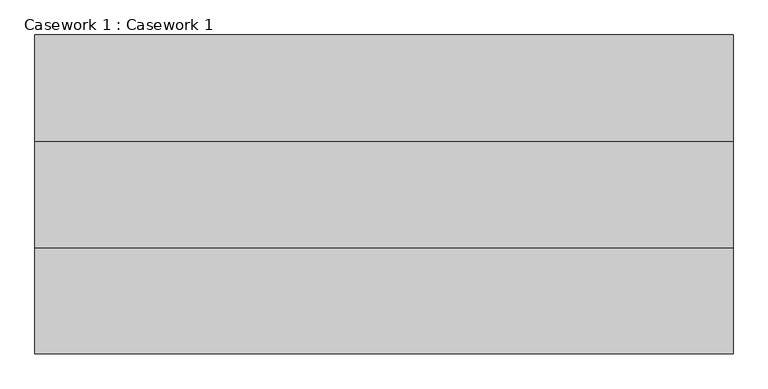
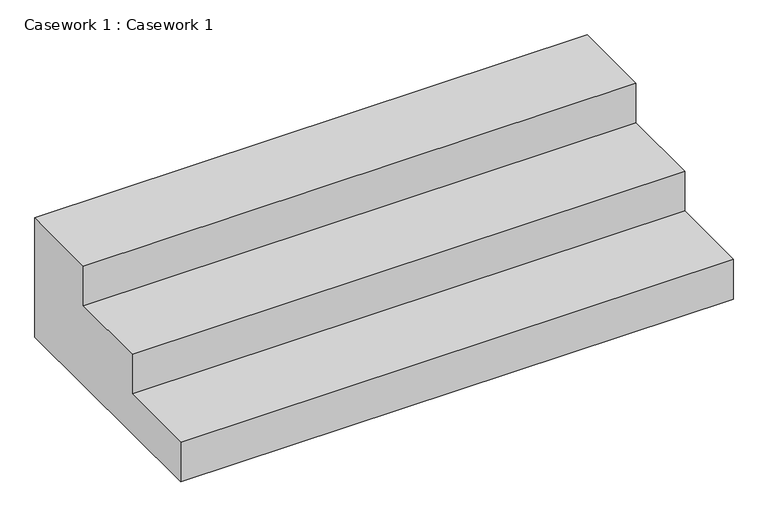
"""IFC4 building model written with IfcOpenShell, lengths in millimetres: furniture geometry, Casework 1 : Casework 1."""

from ifc_helpers import new_model, si_unit, frame, origin, place, context, project, spatial, polyline, outline, extrude, source, transform, mapped, element, save


def casework_1_casework_1_50447f05(model_context):
    return source(origin(), model_context, "Body", "SweptSolid", [
        extrude(outline(polyline([(2155.1965218, 457.2), (2459.9965218, 457.2), (2459.9965218, 0.0), (1545.5965218, 0.0), (1545.5965218, 152.4), (1850.3965218, 152.4), (1850.3965218, 304.8), (2155.1965218, 304.8), (2155.1965218, 457.2)])), frame((-9890.3237872, 0.0, 0.0), z_axis=(1.0, 0.0, 0.0), x_axis=(0.0, 1.0, 0.0)), (0.0, 0.0, 1.0), 2001.725458),
    ])


if __name__ == "__main__":
    model = new_model("IFC4")
    model_context = context("Model", 3, world=origin())
    ifc_project = project(units=[si_unit("LENGTHUNIT", "METRE", prefix="MILLI")], contexts=[model_context])
    site = spatial("IfcSite", under=ifc_project)
    building = spatial("IfcBuilding", under=site)
    placement = place(None, origin())
    casework_1_casework_1_shape = casework_1_casework_1_50447f05(model_context)
    element("IfcFurniture", 1, ObjectType="Casework 1 : Casework 1", at=placement, inside=building, context=model_context, shape_type="MappedRepresentation", body=[
        mapped(casework_1_casework_1_shape, transform((0.0, 0.0, 0.0), x_axis=(1.0, 0.0, 0.0), y_axis=(0.0, 1.0, 0.0), z_axis=(0.0, 0.0, 1.0))),
    ])
    save(model, "model.ifc")

# Revit data of these elements
# Element 1 (IfcFurniture, "Casework 1 : Casework 1")
#   Materials on its faces: "Concrete, Cast-in-Place gray"
# Materials
#   "Concrete, Cast-in-Place gray": class "Concrete", colour RGB 192 192 192, transparency 0, Description = "Cast-in-place concrete", Cost = 0
